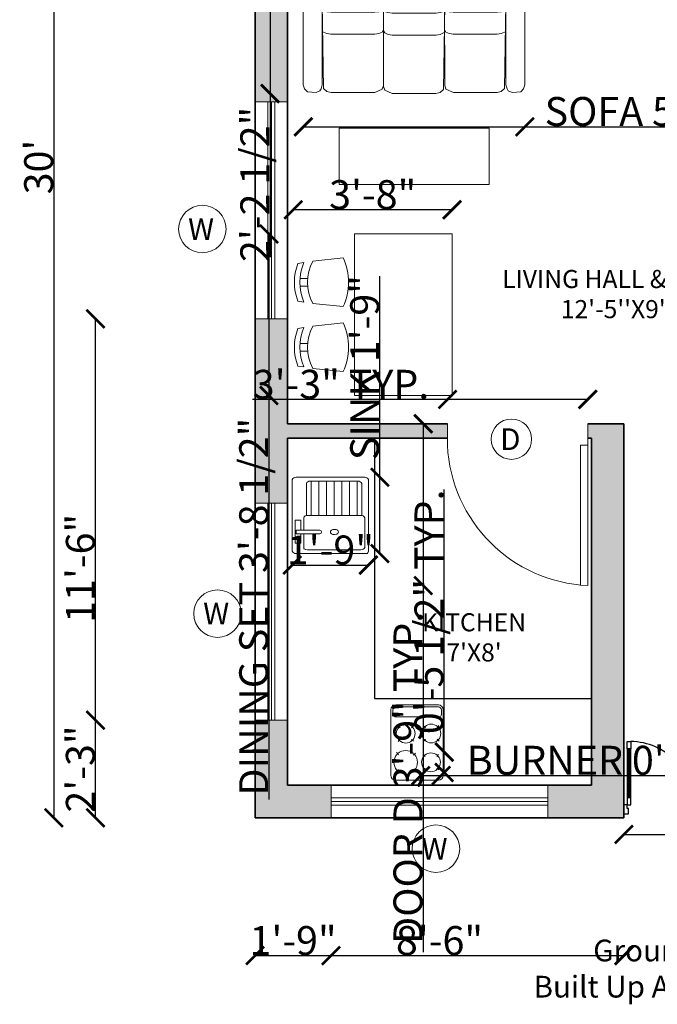
# Model space of a CAD drawing. Units: inches. Extents: x 2163 to 2555, y 1763 to 2232.
# Tile 1 of 3: x 2163 to 2339, y 1763 to 2035. Entities that reach past the tile are written whole.
import ezdxf

# ---------------------------------------------------------------- set-up
doc = ezdxf.new("R2010")
doc.units = ezdxf.units.IN
for name, color, linetype, lineweight in [('A-ANNO-DIMS', 2, 'Continuous', 18), ('A-ANNO-SYMB', 7, 'Continuous', 18), ('A-ANNO-TEXT', 7, 'Continuous', 18), ('A-AREA-IDEN', 7, 'Continuous', 18), ('A-EQPM', 9, 'Continuous', 18), ('A-FLOR-FIXT', 9, 'Continuous', 18), ('A-FURN', 8, 'Continuous', 18), ('A-WALL-PATT', 8, 'Continuous', 13), ('Doors', 222, 'Continuous', 18), ('Kitchen', 92, 'Continuous', 25), ('Walls', 7, 'Continuous', 35), ('Windows', 150, 'Continuous', 18)]:
    doc.layers.add(name, color=color, linetype=linetype, lineweight=lineweight)
doc.layers.add('A-Glaz', color=92, linetype='Continuous')
doc.layers.add('Main Door', color=150, linetype='Continuous')
doc.styles.get("Standard").update_dxf_attribs({"font": 'arial.ttf'})
doc.dimstyles.get("Standard").update_dxf_attribs({"dimtxt": 8, "dimasz": 5, "dimexe": 0.18, "dimexo": 0.0625, "dimgap": 0.09, "dimtad": 1, "dimdec": 1, "dimzin": 0, "dimdsep": 46, "dimlunit": 4, "dimtxsty": 'Standard', "dimblk": 'ARCHTICK', "dimcen": 0.09, "dimse1": 1, "dimse2": 1, "dimadec": 0, "dimazin": 0, "dimtfac": 1, "dimtdec": 1, "dimtofl": 0, "dimtmove": 0, "dimatfit": 3, "dimfxl": 1, "dimtolj": 1, "dimtzin": 0, "dimarcsym": 0})

# ---------------------------------------------------------------- blocks, each defined once
blk = doc.blocks.new('A$C13CE0A17')
at = {"layer": 'A-Glaz'}
for p, q in [((0.01, 0.61), (0.01, 0.08)), ((0.03, 0.08), (0.03, 0.61))]:
    blk.add_line(p, q, dxfattribs=at)
blk.add_lwpolyline([(1.4, 0.08), (1.4, 0.61), (1.42, 0.61), (1.42, 0.08)], close=True, dxfattribs=at)
at = {"layer": 'Main Door'}
for p, q in [((0, 0.61), (0, 0.69)), ((0, 0.69), (0.04, 0.69)), ((0.04, 0.69), (0.04, 0.61)), ((0, 0.61), (0, 0.08)), ((0.04, 0.61), (0, 0.61)), ((0.04, 0.61), (0, 0.61)), ((0.03, 0.61), (0.01, 0.61)), ((0.04, 0.08), (0.04, 0.61)), ((-0.035, 0), (-0.035, -0.1)), ((0, 0), (-0.035, 0)), ((0, 0.08), (0, 0)), ((0.04, 0.08), (0, 0.08)), ((0, 0.08), (0.04, 0.08)), ((0, 0), (0.04, 0)), ((0, -0.04), (0, 0)), ((0.01, 0.08), (0.03, 0.08)), ((0.04, 0), (0.04, 0.08)), ((-0.035, -0.1), (0.015, -0.1)), ((0.015, -0.04), (0, -0.04)), ((0.015, -0.05), (0.015, -0.04)), ((0.015, -0.1), (0.015, -0.05))]:
    blk.add_line(p, q, dxfattribs=at)
for points in [[(1.39, 0.69), (1.39, 0.61), (1.43, 0.61), (1.43, 0.69)], [(1.39, 0.08), (1.39, 0.61), (1.43, 0.61), (1.43, 0.08)], [(1.39, 0), (1.39, 0.08), (1.43, 0.08), (1.43, 0)], [(1.43, 0), (1.465, 0), (1.465, -0.1), (1.415, -0.1), (1.415, -0.05), (1.415, -0.04), (1.43, -0.04)]]:
    blk.add_lwpolyline(points, close=True, dxfattribs=at)
blk.add_arc((1.387, 0.017), 0.673, 89.7657, 181.4438, dxfattribs=at)
blk.add_ellipse((0.039, 0.051), major_axis=(0.667, -0.122), ratio=0.940794, start_param=0.11153, end_param=1.73917, dxfattribs=at)
blk = doc.blocks.new('S_SINK12')
for p, q in [((0.25, 0.45), (0.25, 0)), ((0.35, 0.45), (0.35, 0)), ((0.45, 0.45), (0.45, 0)), ((0.55, 0.45), (0.55, 0)), ((0.65, 0.45), (0.65, 0)), ((0.75, 0.45), (0.75, 0)), ((0.85, 0.45), (0.85, 0))]:
    blk.add_line(p, q)
for points in [[(0, -0.469), (0, 0.469, -0.310961), (0.05, 0.5), (0.95, 0.5, -0.310466), (1, 0.469), (1, -0.469, -0.414214), (0.969, -0.5), (0.05, -0.5, -0.309971)], [(0.052, -0.195), (0.052, -0.242), (0.362, -0.242, 1), (0.362, -0.195)], [(0.5, -0.217), (0.503, -0.229, 0.107136), (0.516, -0.241, 0.076468), (0.534, -0.249), (0.554, -0.251), (0.575, -0.248, 0.076468), (0.592, -0.241, 0.107136), (0.604, -0.229), (0.608, -0.217), (0.604, -0.205, 0.107136), (0.592, -0.193, 0.076468), (0.575, -0.186), (0.554, -0.183), (0.532, -0.186, 0.076468), (0.516, -0.193, 0.107136), (0.503, -0.205)]]:
    blk.add_lwpolyline(points, format="xyb", close=True)
for points in [[(0.185, -0.001), (0.185, 0.419, -0.310466), (0.235, 0.45), (0.862, 0.45, -0.310466), (0.912, 0.419), (0.912, 0, -0.310466)], [(0.15, -0.195), (0.15, -0.031, -0.310466), (0.2, 0), (0.9, 0, -0.310466), (0.95, -0.031), (0.95, -0.419, -0.310466), (0.9, -0.45), (0.2, -0.45), (0.18, -0.448, -0.071009), (0.165, -0.442, -0.106323), (0.153, -0.432), (0.15, -0.422), (0.151, -0.419)]]:
    blk.add_lwpolyline(points, format="xyb")
for points in [[(0.114, -0.242), (0.114, -0.364), (0.039, -0.364), (0.039, -0.064), (0.114, -0.064), (0.114, -0.195)], [(0.15, -0.419), (0.15, -0.242)]]:
    blk.add_lwpolyline(points)
blk = doc.blocks.new('table-23')
at = {"color": 0, "linetype": 'ByBlock'}
for p, q in [((-0.9, -1.4923), (-0.9, 0)), ((-0.9, 0), (0, 0)), ((0, -1.4923), (0, 0)), ((0.1062, -0.2211), (0.3862, -0.2511)), ((0.4677, -0.2639), (0.5237, -0.2726)), ((0.5049, -0.4111), (0.4347, -0.4111)), ((0.5049, -0.4811), (0.4347, -0.4811)), ((0.4677, -0.6284), (0.5237, -0.6197)), ((0.1062, -0.6711), (0.3862, -0.6411)), ((0.1062, -0.8211), (0.3862, -0.8511)), ((0.4677, -0.8639), (0.5237, -0.8726)), ((0.5049, -1.0111), (0.4347, -1.0111)), ((0.5049, -1.0811), (0.4347, -1.0811)), ((0.1062, -1.2711), (0.3862, -1.2411)), ((0.4677, -1.2284), (0.5237, -1.2197)), ((-0.9, -1.4923), (0, -1.4923))]:
    blk.add_line(p, q, dxfattribs=at)
for centre, radius, start, end in [((0.5875, -0.4461), 0.5312, 154.94238, 205.05762), ((0.031, -0.4461), 0.4053, 331.23721, 28.76279), ((0.0558, -0.4461), 0.4505, 336.13443, 23.86557), ((0.0765, -0.4461), 0.4797, 338.78869, 21.21131), ((0.5875, -1.0461), 0.5312, 154.94238, 205.05762), ((0.031, -1.0461), 0.4053, 331.23721, 28.76279), ((0.0558, -1.0461), 0.4505, 336.13443, 23.86557), ((0.0765, -1.0461), 0.4797, 338.78869, 21.21131)]:
    blk.add_arc(centre, radius, start, end, dxfattribs=at)
blk = doc.blocks.new('AP0B05')
for p, q in [((35, 100), (35, 880)), ((75, 100), (75, 878.9)), ((35, 100), (35, -20)), ((815, 100), (815, -20))]:
    blk.add_line(p, q)
blk.add_lwpolyline([(35, 100), (75, 100)])
blk.add_arc((-2.4, 62.6), 818.3, 2.6212, 87.3788)
blk = doc.blocks.new('12PCOU17')
at = {"color": 0, "linetype": 'ByBlock'}
for points in [[(-34.71, 34.72), (-33.66, 34.31), (-3.27, 34.3), (-1.81, 34.76), (-1.05, 35.2), (-0.38, 36.65), (-0.61, 39.84), (-1.73, 40.94), (-3.27, 41.4), (-33.66, 41.4), (-34.95, 40.5), (-35.65, 39.02), (-35.49, 35.83), (-34.71, 34.72)], [(-1.89, 11.91), (-1.66, 11.91), (-0.35, 14.68), (-0.35, 31.05), (-0.74, 32.58), (-1.89, 33.83), (-33.63, 34.3), (-34.84, 33.63), (-35.43, 32.38), (-35.68, 31), (-35.68, 14.74), (-35.43, 13.36), (-34.66, 11.99), (-33.44, 11.43), (-3, 11.44), (-1.66, 11.91)], [(-31.25, 11.43), (-31.06, 11.84), (-30.6, 13.09), (-30.4, 14.62), (-30.4, 31.12), (-30.6, 32.65), (-31.06, 33.9), (-31.81, 34.3)], [(-23.84, 11.43), (-22.99, 11.9), (-22.46, 13.15), (-22.23, 14.67), (-22.23, 31.07), (-22.46, 32.59), (-22.99, 33.84), (-23.12, 34.3)], [(-1.54, -10.96), (-1.31, -10.96), (0, -8.19), (0, 8.19), (-0.39, 9.71), (-1.54, 10.96), (-33.28, 11.44), (-34.5, 10.77), (-35.08, 9.51), (-35.33, 8.14), (-35.33, -8.13), (-35.08, -9.51), (-34.31, -10.87), (-33.1, -11.44), (-2.65, -11.43), (-1.31, -10.96)], [(-30.9, -11.44), (-30.72, -11.02), (-30.25, -9.77), (-30.05, -8.25), (-30.05, 8.26), (-30.25, 9.78), (-30.72, 11.03), (-31.47, 11.44)], [(-23.49, -11.44), (-22.64, -10.96), (-22.11, -9.72), (-21.88, -8.19), (-21.88, 8.2), (-22.11, 9.73), (-22.64, 10.97), (-22.77, 11.44)], [(-1.89, -11.91), (-1.66, -11.91), (-0.35, -14.68), (-0.35, -31.05), (-0.74, -32.58), (-1.89, -33.83), (-33.63, -34.3), (-34.84, -33.63), (-35.43, -32.38), (-35.68, -31), (-35.68, -14.74), (-35.43, -13.36), (-34.66, -11.99), (-33.44, -11.43), (-3, -11.44), (-1.66, -11.91)], [(-31.25, -11.43), (-31.06, -11.84), (-30.6, -13.09), (-30.4, -14.62), (-30.4, -31.12), (-30.6, -32.65), (-31.06, -33.9), (-31.81, -34.3)], [(-23.84, -11.43), (-22.99, -11.9), (-22.46, -13.15), (-22.23, -14.67), (-22.23, -31.07), (-22.46, -32.59), (-22.99, -33.84), (-23.12, -34.3)], [(-34.71, -34.72), (-33.66, -34.31), (-3.27, -34.3), (-1.81, -34.76), (-1.05, -35.2), (-0.38, -36.65), (-0.61, -39.84), (-1.73, -40.94), (-3.27, -41.4), (-33.66, -41.4), (-34.95, -40.5), (-35.65, -39.02), (-35.49, -35.83), (-34.71, -34.72)]]:
    blk.add_lwpolyline(points, dxfattribs=at)
blk = doc.blocks.new('_ArchTick')
at = {"color": 0, "linetype": 'ByBlock', "const_width": 0.15}
blk.add_lwpolyline([(-0.5, -0.5), (0.5, 0.5)], dxfattribs=at)
blk = doc.blocks.new('*D12')
at = {"layer": 'A-ANNO-DIMS', "color": 0, "lineweight": -2, "transparency": 16777216}
blk.add_line((2172.33, 2174.5), (2172.33, 1814.5), dxfattribs=at)
at = {"layer": 'Defpoints', "color": 0, "transparency": 16777216}
for p in [(2228.01, 2174.5), (2172.33, 1814.5), (2228.01, 1814.5)]:
    blk.add_point(p, dxfattribs=at)
at = {"layer": 'A-ANNO-DIMS', "color": 0, "lineweight": -2, "transparency": 16777216, "xscale": 5, "yscale": 5, "zscale": 5}
for p, rotation in [((2172.33, 2174.5), 90), ((2172.33, 1814.5), 270)]:
    blk.add_blockref('_ArchTick', p, dxfattribs=dict(at, rotation=rotation))
at = {"layer": 'A-ANNO-DIMS', "color": 0, "transparency": 16777216, "insert": (2168.15, 1994.5), "char_height": 8, "attachment_point": 5, "rotation": 90}
blk.add_mtext("\\A1;30'", dxfattribs=at)
blk = doc.blocks.new('WIN-60IN')
for p, q in [((0, 5.5), (60, 5.5)), ((0, 4.5), (60, 4.5)), ((0, 3.5), (60, 3.5))]:
    blk.add_line(p, q)
blk.add_lwpolyline([(0, 9), (60, 9), (60, 0), (0, 0)], close=True)
blk = doc.blocks.new('TAG-WINDOW-W')
blk.add_circle((6.57, 6.57), 6.57)
blk.add_text('W', height=6).set_placement((2.61, 3.57))
blk = doc.blocks.new('TAG-DOOR-D')
blk.add_circle((5.58, 5.58), 5.58)
blk.add_text('D', height=6).set_placement((2.46, 2.58))
blk = doc.blocks.new('COOKTOP-BURNER')
for p, q in [((0.44, 4.72), (1.01, 4.18)), ((4.72, 4.76), (4.18, 4.18)), ((0.47, 0.44), (1.02, 1.01)), ((4.76, 0.47), (4.18, 1.02))]:
    blk.add_line(p, q)
for start, end in [(138.017, 221.983), (48.017, 131.983), (318.017, 41.983), (228.017, 311.983)]:
    blk.add_arc((2.6, 2.6), 2.6, start, end)
blk = doc.blocks.new('*D20')
at = {"layer": 'A-ANNO-DIMS', "color": 0, "lineweight": -2, "transparency": 16777216}
for p, q in [((2274.51, 1923.5), (2274.51, 1878.74)), ((2274.51, 1878.74), (2274.51, 1777.39))]:
    blk.add_line(p, q, dxfattribs=at)
at = {"layer": 'Defpoints', "color": 0, "transparency": 16777216}
for p in [(2281.23, 1923.5), (2274.51, 1878.74), (2281.23, 1878.74)]:
    blk.add_point(p, dxfattribs=at)
at = {"layer": 'A-ANNO-DIMS', "color": 0, "lineweight": -2, "transparency": 16777216, "xscale": 5, "yscale": 5, "zscale": 5}
for p, rotation in [((2274.51, 1923.5), 90), ((2274.51, 1878.74), 270)]:
    blk.add_blockref('_ArchTick', p, dxfattribs=dict(at, rotation=rotation))
at = {"layer": 'A-ANNO-DIMS', "color": 0, "transparency": 16777216, "insert": (2270.28, 1825.56), "char_height": 8, "attachment_point": 5, "rotation": 90}
blk.add_mtext('\\A1;DOOR D 3\'-9" TYP.', dxfattribs=at)
blk = doc.blocks.new('*D21')
at = {"layer": 'A-ANNO-DIMS', "color": 0, "lineweight": -2, "transparency": 16777216}
for p, q in [((2281.23, 1930.22), (2227.29, 1930.22)), ((2320.02, 1930.22), (2281.23, 1930.22))]:
    blk.add_line(p, q, dxfattribs=at)
at = {"layer": 'Defpoints', "color": 0, "transparency": 16777216}
for p in [(2281.23, 1930.22), (2281.23, 1923.5), (2320.02, 1923.5)]:
    blk.add_point(p, dxfattribs=at)
at = {"layer": 'A-ANNO-DIMS', "color": 0, "lineweight": -2, "transparency": 16777216, "xscale": 5, "yscale": 5, "zscale": 5, "rotation": 180}
blk.add_blockref('_ArchTick', (2281.23, 1930.22), dxfattribs=at)
at = {"layer": 'A-ANNO-DIMS', "color": 0, "lineweight": -2, "transparency": 16777216, "xscale": 5, "yscale": 5, "zscale": 5}
blk.add_blockref('_ArchTick', (2320.02, 1930.22), dxfattribs=at)
at = {"layer": 'A-ANNO-DIMS', "color": 0, "transparency": 16777216, "insert": (2251.76, 1934.4), "char_height": 8, "attachment_point": 5}
blk.add_mtext('\\A1;3\'-3" TYP.', dxfattribs=at)
blk = doc.blocks.new('*D24')
at = {"layer": 'A-ANNO-DIMS', "color": 0, "lineweight": -2, "transparency": 16777216}
for p, q in [((2273.83, 1826.19), (2279.47, 1826.19)), ((2279.47, 1826.19), (2402, 1826.19))]:
    blk.add_line(p, q, dxfattribs=at)
at = {"layer": 'Defpoints', "color": 0, "transparency": 16777216}
for p in [(2273.83, 1827.04), (2279.47, 1827.04), (2279.47, 1826.19)]:
    blk.add_point(p, dxfattribs=at)
at = {"layer": 'A-ANNO-DIMS', "color": 0, "lineweight": -2, "transparency": 16777216, "xscale": 5, "yscale": 5, "zscale": 5, "rotation": 180}
blk.add_blockref('_ArchTick', (2273.83, 1826.19), dxfattribs=at)
at = {"layer": 'A-ANNO-DIMS', "color": 0, "lineweight": -2, "transparency": 16777216, "xscale": 5, "yscale": 5, "zscale": 5}
blk.add_blockref('_ArchTick', (2279.47, 1826.19), dxfattribs=at)
at = {"layer": 'A-ANNO-DIMS', "color": 0, "transparency": 16777216, "insert": (2343.23, 1830.42), "char_height": 8, "attachment_point": 5}
blk.add_mtext('\\A1;BURNER 0\'-5 1/2" TYP.', dxfattribs=at)
blk = doc.blocks.new('*D25')
at = {"layer": 'A-ANNO-DIMS', "color": 0, "lineweight": -2, "transparency": 16777216}
for p, q in [((2280.31, 1832.68), (2280.31, 1905.27)), ((2280.31, 1827.04), (2280.31, 1832.68))]:
    blk.add_line(p, q, dxfattribs=at)
at = {"layer": 'Defpoints', "color": 0, "transparency": 16777216}
for p in [(2279.47, 1832.68), (2280.31, 1832.68), (2279.47, 1827.04)]:
    blk.add_point(p, dxfattribs=at)
at = {"layer": 'A-ANNO-DIMS', "color": 0, "lineweight": -2, "transparency": 16777216, "xscale": 5, "yscale": 5, "zscale": 5}
for p, rotation in [((2280.31, 1832.68), 90), ((2280.31, 1827.04), 270)]:
    blk.add_blockref('_ArchTick', p, dxfattribs=dict(at, rotation=rotation))
at = {"layer": 'A-ANNO-DIMS', "color": 0, "transparency": 16777216, "insert": (2276.09, 1871.47), "char_height": 8, "attachment_point": 5, "rotation": 90}
blk.add_mtext('\\A1;0\'-5 1/2" TYP.', dxfattribs=at)
blk = doc.blocks.new('*D32')
at = {"layer": 'A-ANNO-DIMS', "color": 0, "lineweight": -2, "transparency": 16777216}
for p, q in [((2330.01, 1809.91), (2368.01, 1809.91)), ((2368.01, 1809.91), (2471.65, 1809.91))]:
    blk.add_line(p, q, dxfattribs=at)
at = {"layer": 'Defpoints', "color": 0, "transparency": 16777216}
for p in [(2330.01, 1815.61), (2368.01, 1815.61), (2368.01, 1809.91)]:
    blk.add_point(p, dxfattribs=at)
at = {"layer": 'A-ANNO-DIMS', "color": 0, "lineweight": -2, "transparency": 16777216, "xscale": 5, "yscale": 5, "zscale": 5, "rotation": 180}
blk.add_blockref('_ArchTick', (2330.01, 1809.91), dxfattribs=at)
at = {"layer": 'A-ANNO-DIMS', "color": 0, "lineweight": -2, "transparency": 16777216, "xscale": 5, "yscale": 5, "zscale": 5}
blk.add_blockref('_ArchTick', (2368.01, 1809.91), dxfattribs=at)
at = {"layer": 'A-ANNO-DIMS', "color": 0, "transparency": 16777216, "insert": (2422.33, 1814.14), "char_height": 8, "attachment_point": 5}
blk.add_mtext('\\A1;ENTRY DOOR 3\'-2"', dxfattribs=at)
blk = doc.blocks.new('*D34')
at = {"layer": 'A-ANNO-DIMS', "color": 0, "lineweight": -2, "transparency": 16777216}
for p, q in [((2262.54, 1908.7), (2262.54, 1964.3)), ((2262.54, 1887.57), (2262.54, 1908.7))]:
    blk.add_line(p, q, dxfattribs=at)
at = {"layer": 'Defpoints', "color": 0, "transparency": 16777216}
for p in [(2259.37, 1908.7), (2262.54, 1908.7), (2259.37, 1887.57)]:
    blk.add_point(p, dxfattribs=at)
at = {"layer": 'A-ANNO-DIMS', "color": 0, "lineweight": -2, "transparency": 16777216, "xscale": 5, "yscale": 5, "zscale": 5}
for p, rotation in [((2262.54, 1908.7), 90), ((2262.54, 1887.57), 270)]:
    blk.add_blockref('_ArchTick', p, dxfattribs=dict(at, rotation=rotation))
at = {"layer": 'A-ANNO-DIMS', "color": 0, "transparency": 16777216, "insert": (2258.32, 1939), "char_height": 8, "attachment_point": 5, "rotation": 90}
blk.add_mtext('\\A1;SINK 1\'-9"', dxfattribs=at)
blk = doc.blocks.new('*D35')
at = {"layer": 'A-ANNO-DIMS', "color": 0, "lineweight": -2, "transparency": 16777216}
blk.add_line((2238.28, 1884.4), (2259.37, 1884.4), dxfattribs=at)
at = {"layer": 'Defpoints', "color": 0, "transparency": 16777216}
for p in [(2238.28, 1887.57), (2259.37, 1887.57), (2259.37, 1884.4)]:
    blk.add_point(p, dxfattribs=at)
at = {"layer": 'A-ANNO-DIMS', "color": 0, "lineweight": -2, "transparency": 16777216, "xscale": 5, "yscale": 5, "zscale": 5, "rotation": 180}
blk.add_blockref('_ArchTick', (2238.28, 1884.4), dxfattribs=at)
at = {"layer": 'A-ANNO-DIMS', "color": 0, "lineweight": -2, "transparency": 16777216, "xscale": 5, "yscale": 5, "zscale": 5}
blk.add_blockref('_ArchTick', (2259.37, 1884.4), dxfattribs=at)
at = {"layer": 'A-ANNO-DIMS', "color": 0, "transparency": 16777216, "insert": (2248.83, 1888.57), "char_height": 8, "attachment_point": 5}
blk.add_mtext('\\A1;1\'-9"', dxfattribs=at)
blk = doc.blocks.new('*D36')
at = {"layer": 'A-ANNO-DIMS', "color": 0, "lineweight": -2, "transparency": 16777216}
for p, q in [((2231.85, 1975.97), (2231.85, 1931.28)), ((2231.85, 1931.28), (2231.85, 1819.53))]:
    blk.add_line(p, q, dxfattribs=at)
at = {"layer": 'Defpoints', "color": 0, "transparency": 16777216}
for p in [(2238.56, 1975.97), (2231.85, 1931.28), (2238.56, 1931.28)]:
    blk.add_point(p, dxfattribs=at)
at = {"layer": 'A-ANNO-DIMS', "color": 0, "lineweight": -2, "transparency": 16777216, "xscale": 5, "yscale": 5, "zscale": 5}
for p, rotation in [((2231.85, 1975.97), 90), ((2231.85, 1931.28), 270)]:
    blk.add_blockref('_ArchTick', p, dxfattribs=dict(at, rotation=rotation))
at = {"layer": 'A-ANNO-DIMS', "color": 0, "transparency": 16777216, "insert": (2227.62, 1872.9), "char_height": 8, "attachment_point": 5, "rotation": 90}
blk.add_mtext('\\A1;DINING SET 3\'-8 1/2"', dxfattribs=at)
blk = doc.blocks.new('*D37')
at = {"layer": 'A-ANNO-DIMS', "color": 0, "lineweight": -2, "transparency": 16777216}
blk.add_line((2282.49, 1982.67), (2238.56, 1982.67), dxfattribs=at)
at = {"layer": 'Defpoints', "color": 0, "transparency": 16777216}
for p in [(2238.56, 1982.67), (2238.56, 1975.97), (2282.49, 1975.97)]:
    blk.add_point(p, dxfattribs=at)
at = {"layer": 'A-ANNO-DIMS', "color": 0, "lineweight": -2, "transparency": 16777216, "xscale": 5, "yscale": 5, "zscale": 5, "rotation": 180}
blk.add_blockref('_ArchTick', (2238.56, 1982.67), dxfattribs=at)
at = {"layer": 'A-ANNO-DIMS', "color": 0, "lineweight": -2, "transparency": 16777216, "xscale": 5, "yscale": 5, "zscale": 5}
blk.add_blockref('_ArchTick', (2282.49, 1982.67), dxfattribs=at)
at = {"layer": 'A-ANNO-DIMS', "color": 0, "transparency": 16777216, "insert": (2260.53, 1986.85), "char_height": 8, "attachment_point": 5}
blk.add_mtext('\\A1;3\'-8"', dxfattribs=at)
blk = doc.blocks.new('*D38')
at = {"layer": 'A-ANNO-DIMS', "color": 0, "lineweight": -2, "transparency": 16777216}
for p, q in [((2241.35, 2005.61), (2302.62, 2005.61)), ((2302.62, 2005.61), (2381.2, 2005.61))]:
    blk.add_line(p, q, dxfattribs=at)
at = {"layer": 'Defpoints', "color": 0, "transparency": 16777216}
for p in [(2241.35, 2014.8), (2302.62, 2014.8), (2302.62, 2005.61)]:
    blk.add_point(p, dxfattribs=at)
at = {"layer": 'A-ANNO-DIMS', "color": 0, "lineweight": -2, "transparency": 16777216, "xscale": 5, "yscale": 5, "zscale": 5, "rotation": 180}
blk.add_blockref('_ArchTick', (2241.35, 2005.61), dxfattribs=at)
at = {"layer": 'A-ANNO-DIMS', "color": 0, "lineweight": -2, "transparency": 16777216, "xscale": 5, "yscale": 5, "zscale": 5}
blk.add_blockref('_ArchTick', (2302.62, 2005.61), dxfattribs=at)
at = {"layer": 'A-ANNO-DIMS', "color": 0, "transparency": 16777216, "insert": (2344.41, 2009.84), "char_height": 8, "attachment_point": 5}
blk.add_mtext('\\A1;SOFA 5\'-1 1/2"', dxfattribs=at)
blk = doc.blocks.new('*D39')
at = {"layer": 'A-ANNO-DIMS', "color": 0, "lineweight": -2, "transparency": 16777216}
for p, q in [((2232.15, 2041.21), (2232.15, 2014.8)), ((2232.15, 2014.8), (2232.15, 1969.58))]:
    blk.add_line(p, q, dxfattribs=at)
at = {"layer": 'Defpoints', "color": 0, "transparency": 16777216}
for p in [(2241.35, 2041.21), (2232.15, 2014.8), (2241.35, 2014.8)]:
    blk.add_point(p, dxfattribs=at)
at = {"layer": 'A-ANNO-DIMS', "color": 0, "lineweight": -2, "transparency": 16777216, "xscale": 5, "yscale": 5, "zscale": 5}
for p, rotation in [((2232.15, 2041.21), 90), ((2232.15, 2014.8), 270)]:
    blk.add_blockref('_ArchTick', p, dxfattribs=dict(at, rotation=rotation))
at = {"layer": 'A-ANNO-DIMS', "color": 0, "transparency": 16777216, "insert": (2227.93, 1989.69), "char_height": 8, "attachment_point": 5, "rotation": 90}
blk.add_mtext('\\A1;2\'-2 1/2"', dxfattribs=at)
blk = doc.blocks.new('*D45')
at = {"layer": 'A-ANNO-DIMS', "color": 0, "lineweight": -2, "transparency": 16777216}
blk.add_line((2228.01, 1776.39), (2249.01, 1776.39), dxfattribs=at)
at = {"layer": 'Defpoints', "color": 0, "transparency": 16777216}
for p in [(2228.01, 1814.5), (2249.01, 1814.5), (2249.01, 1776.39)]:
    blk.add_point(p, dxfattribs=at)
at = {"layer": 'A-ANNO-DIMS', "color": 0, "lineweight": -2, "transparency": 16777216, "xscale": 5, "yscale": 5, "zscale": 5, "rotation": 180}
blk.add_blockref('_ArchTick', (2228.01, 1776.39), dxfattribs=at)
at = {"layer": 'A-ANNO-DIMS', "color": 0, "lineweight": -2, "transparency": 16777216, "xscale": 5, "yscale": 5, "zscale": 5}
blk.add_blockref('_ArchTick', (2249.01, 1776.39), dxfattribs=at)
at = {"layer": 'A-ANNO-DIMS', "color": 0, "transparency": 16777216, "insert": (2238.51, 1780.56), "char_height": 8, "attachment_point": 5}
blk.add_mtext('\\A1;1\'-9"', dxfattribs=at)
blk = doc.blocks.new('*D46')
at = {"layer": 'A-ANNO-DIMS', "color": 0, "lineweight": -2, "transparency": 16777216}
blk.add_line((2228.01, 1776.39), (2330.01, 1776.39), dxfattribs=at)
at = {"layer": 'Defpoints', "color": 0, "transparency": 16777216}
for p in [(2228.01, 1814.5), (2330.01, 1814.5), (2330.01, 1776.39)]:
    blk.add_point(p, dxfattribs=at)
at = {"layer": 'A-ANNO-DIMS', "color": 0, "lineweight": -2, "transparency": 16777216, "xscale": 5, "yscale": 5, "zscale": 5, "rotation": 180}
blk.add_blockref('_ArchTick', (2228.01, 1776.39), dxfattribs=at)
at = {"layer": 'A-ANNO-DIMS', "color": 0, "lineweight": -2, "transparency": 16777216, "xscale": 5, "yscale": 5, "zscale": 5}
blk.add_blockref('_ArchTick', (2330.01, 1776.39), dxfattribs=at)
at = {"layer": 'A-ANNO-DIMS', "color": 0, "transparency": 16777216, "insert": (2279.01, 1780.56), "char_height": 8, "attachment_point": 5}
blk.add_mtext('\\A1;8\'-6"', dxfattribs=at)
blk = doc.blocks.new('*D47')
at = {"layer": 'A-ANNO-DIMS', "color": 0, "lineweight": -2, "transparency": 16777216}
blk.add_line((2183.86, 1814.5), (2183.86, 1841.5), dxfattribs=at)
at = {"layer": 'Defpoints', "color": 0, "transparency": 16777216}
for p in [(2183.86, 1841.5), (2228.01, 1841.5), (2228.01, 1814.5)]:
    blk.add_point(p, dxfattribs=at)
at = {"layer": 'A-ANNO-DIMS', "color": 0, "lineweight": -2, "transparency": 16777216, "xscale": 5, "yscale": 5, "zscale": 5}
for p, rotation in [((2183.86, 1841.5), 90), ((2183.86, 1814.5), 270)]:
    blk.add_blockref('_ArchTick', p, dxfattribs=dict(at, rotation=rotation))
at = {"layer": 'A-ANNO-DIMS', "color": 0, "transparency": 16777216, "insert": (2179.68, 1828), "char_height": 8, "attachment_point": 5, "rotation": 90}
blk.add_mtext('\\A1;2\'-3"', dxfattribs=at)
blk = doc.blocks.new('*D48')
at = {"layer": 'A-ANNO-DIMS', "color": 0, "lineweight": -2, "transparency": 16777216}
blk.add_line((2183.86, 1814.5), (2183.86, 1952.5), dxfattribs=at)
at = {"layer": 'Defpoints', "color": 0, "transparency": 16777216}
for p in [(2183.86, 1952.5), (2228.01, 1952.5), (2228.01, 1814.5)]:
    blk.add_point(p, dxfattribs=at)
at = {"layer": 'A-ANNO-DIMS', "color": 0, "lineweight": -2, "transparency": 16777216, "xscale": 5, "yscale": 5, "zscale": 5}
for p, rotation in [((2183.86, 1952.5), 90), ((2183.86, 1814.5), 270)]:
    blk.add_blockref('_ArchTick', p, dxfattribs=dict(at, rotation=rotation))
at = {"layer": 'A-ANNO-DIMS', "color": 0, "transparency": 16777216, "insert": (2179.68, 1883.5), "char_height": 8, "attachment_point": 5, "rotation": 90}
blk.add_mtext('\\A1;11\'-6"', dxfattribs=at)
blk = doc.blocks.new('*D55')
at = {"layer": 'A-ANNO-DIMS', "color": 0, "lineweight": -2, "transparency": 16777216}
blk.add_line((2237.01, 2215.35), (2261.01, 2215.35), dxfattribs=at)
at = {"layer": 'Defpoints', "color": 0, "transparency": 16777216}
for p in [(2261.01, 2215.35), (2237.01, 1919.5), (2261.01, 1919.5)]:
    blk.add_point(p, dxfattribs=at)
at = {"layer": 'A-ANNO-DIMS', "color": 0, "lineweight": -2, "transparency": 16777216, "xscale": 5, "yscale": 5, "zscale": 5, "rotation": 180}
blk.add_blockref('_ArchTick', (2237.01, 2215.35), dxfattribs=at)
at = {"layer": 'A-ANNO-DIMS', "color": 0, "lineweight": -2, "transparency": 16777216, "xscale": 5, "yscale": 5, "zscale": 5}
blk.add_blockref('_ArchTick', (2261.01, 2215.35), dxfattribs=at)
at = {"layer": 'A-ANNO-DIMS', "color": 0, "transparency": 16777216, "insert": (2249.01, 2219.53), "char_height": 8, "attachment_point": 5}
blk.add_mtext('\\A1;2\'-0"', dxfattribs=at)
blk = doc.blocks.new('*D58')
at = {"layer": 'A-ANNO-DIMS', "color": 0, "lineweight": -2, "transparency": 16777216}
for p, q in [((2265.57, 2215.35), (2280.07, 2215.35)), ((2280.07, 2215.35), (2324.4, 2215.35))]:
    blk.add_line(p, q, dxfattribs=at)
at = {"layer": 'Defpoints', "color": 0, "transparency": 16777216}
for p in [(2280.07, 2215.35), (2265.57, 1844.36), (2280.07, 1844.36)]:
    blk.add_point(p, dxfattribs=at)
at = {"layer": 'A-ANNO-DIMS', "color": 0, "lineweight": -2, "transparency": 16777216, "xscale": 5, "yscale": 5, "zscale": 5, "rotation": 180}
blk.add_blockref('_ArchTick', (2265.57, 2215.35), dxfattribs=at)
at = {"layer": 'A-ANNO-DIMS', "color": 0, "lineweight": -2, "transparency": 16777216, "xscale": 5, "yscale": 5, "zscale": 5}
blk.add_blockref('_ArchTick', (2280.07, 2215.35), dxfattribs=at)
at = {"layer": 'A-ANNO-DIMS', "color": 0, "transparency": 16777216, "insert": (2304.73, 2219.58), "char_height": 8, "attachment_point": 5}
blk.add_mtext('\\A1;1\'-2 1/2"', dxfattribs=at)
blk = doc.blocks.new('*D59')
at = {"layer": 'A-ANNO-DIMS', "color": 0, "lineweight": -2, "transparency": 16777216}
blk.add_line((2509.31, 1824.94), (2509.31, 1845.73), dxfattribs=at)
at = {"layer": 'Defpoints', "color": 0, "transparency": 16777216}
for p in [(2278.7, 1845.73), (2509.31, 1845.73), (2278.7, 1824.94)]:
    blk.add_point(p, dxfattribs=at)
at = {"layer": 'A-ANNO-DIMS', "color": 0, "lineweight": -2, "transparency": 16777216, "xscale": 5, "yscale": 5, "zscale": 5}
for p, rotation in [((2509.31, 1845.73), 90), ((2509.31, 1824.94), 270)]:
    blk.add_blockref('_ArchTick', p, dxfattribs=dict(at, rotation=rotation))
at = {"layer": 'A-ANNO-DIMS', "color": 0, "transparency": 16777216, "insert": (2505.14, 1835.33), "char_height": 8, "attachment_point": 5, "rotation": 90}
blk.add_mtext('\\A1;1\'-9"', dxfattribs=at)

msp = doc.modelspace()

# ---------------------------------------------------------------- hatches: boundary and pattern name
at = {"layer": 'A-WALL-PATT', "transparency": 33554585}
h = msp.add_hatch(color=256, dxfattribs=at)
h.dxf.hatch_style = 1
h.paths.add_polyline_path([(2261.51, 2174.5), (2228.01, 2174.5), (2228.01, 2135.5), (2237.01, 2135.5), (2237.01, 2165.5), (2261.51, 2165.5)])
h.paths.add_polyline_path([(2237.01, 2075.5), (2228.01, 2075.5), (2228.01, 2012.5), (2237.01, 2012.5), (2237.01, 2041.5), (2306.96, 2041.5), (2306.96, 2045.5), (2237.01, 2045.5)])
h.paths.add_polyline_path([(2237.01, 1952.5), (2228.01, 1952.5), (2228.01, 1901.5), (2237.01, 1901.5), (2237.01, 1919.5), (2281.23, 1919.5), (2281.23, 1923.5), (2237.01, 1923.5)])
h.paths.add_polyline_path([(2237.01, 1841.5), (2228.01, 1841.5), (2228.01, 1814.5), (2249.01, 1814.5), (2249.01, 1823.5), (2237.01, 1823.5)])
h.paths.add_polyline_path([(2330.01, 1923.5), (2320.02, 1923.5), (2320.02, 1919.5), (2321.01, 1919.5), (2321.01, 1823.5), (2309.01, 1823.5), (2309.01, 1814.5), (2330.01, 1814.5)])
h.paths.add_polyline_path([(2468.01, 1855.84), (2459.01, 1855.84), (2459.01, 1823.5), (2368.01, 1823.5), (2368.01, 1814.5), (2468.01, 1814.5)])
h.paths.add_polyline_path([(2468.01, 1949.34), (2459.01, 1949.34), (2459.01, 1923.5), (2390.01, 1923.5), (2390.01, 2001.5), (2391.3, 2001.5), (2391.3, 2005.5), (2386.01, 2005.5), (2386.01, 1923.5), (2368.01, 1923.5), (2368.01, 1914.5), (2459.01, 1914.5), (2459.01, 1882.16), (2468.01, 1882.16)])
h.paths.add_polyline_path([(2468.01, 2077.97), (2459.01, 2077.97), (2459.01, 2045.5), (2389.06, 2045.5), (2389.06, 2041.5), (2459.01, 2041.5), (2459.01, 2005.5), (2423.94, 2005.5), (2423.94, 2001.5), (2459.01, 2001.5), (2459.01, 1975.66), (2468.01, 1975.66)])
h.paths.add_polyline_path([(2468.01, 2174.5), (2434.51, 2174.5), (2434.51, 2165.5), (2450.4, 2165.5), (2459.01, 2165.5), (2459.01, 2137.97), (2468.01, 2137.97)])

# ---------------------------------------------------------------- linework, layer by layer
at = {"layer": 'A-EQPM'}
for p, q in [((2265.57, 1844.36), (2265.57, 1826.3)), ((2266.11, 1844.36), (2266.11, 1842.99)), ((2278.7, 1845.73), (2266.93, 1845.73)), ((2278.7, 1845.18), (2266.93, 1845.18)), ((2279.52, 1842.99), (2279.52, 1844.36)), ((2280.07, 1826.3), (2280.07, 1844.36)), ((2266.66, 1842.45), (2278.97, 1842.45)), ((2267.1, 1832.53), (2267.71, 1831.88)), ((2272.33, 1832.43), (2271.69, 1831.83)), ((2267.01, 1827.29), (2267.65, 1827.9)), ((2272.24, 1827.2), (2271.63, 1827.84)), ((2266.93, 1824.94), (2278.7, 1824.94))]:
    msp.add_line(p, q, dxfattribs=at)
for centre, radius, start, end in [((2266.93, 1844.36), 1.37, 90, 180), ((2266.93, 1844.36), 0.821, 90, 180), ((2278.7, 1844.36), 1.37, 0, 90), ((2278.7, 1844.36), 0.821, 0, 90), ((2266.66, 1842.99), 0.547, 180, 270), ((2278.97, 1842.99), 0.547, 270, 0), ((2269.67, 1829.86), 3.26, 48.017, 131.983), ((2269.67, 1829.86), 3.26, 138.017, 221.983), ((2269.67, 1829.86), 3.26, 318.017, 41.983), ((2269.67, 1829.86), 3.26, 228.017, 311.983), ((2266.93, 1826.3), 1.37, 180, 270), ((2278.7, 1826.3), 1.37, 270, 0)]:
    msp.add_arc(centre, radius, start, end, dxfattribs=at)
at = {"layer": 'A-FURN'}
msp.add_lwpolyline([(2251.24, 2005.19), (2292.79, 2005.19), (2292.79, 1989.62), (2251.24, 1989.62)], close=True, dxfattribs=at)
at = {"layer": 'Kitchen'}
for p, q in [((2261.01, 1919.5), (2261.01, 1847.5)), ((2261.01, 1847.5), (2321.01, 1847.5))]:
    msp.add_line(p, q, dxfattribs=at)
at = {"layer": 'Walls'}
for p, q in [((2228.01, 2174.5), (2228.01, 1814.5)), ((2237.01, 2041.5), (2237.01, 1923.5)), ((2237.01, 1923.5), (2281.23, 1923.5)), ((2320.02, 1923.5), (2330.01, 1923.5)), ((2330.01, 1923.5), (2330.01, 1814.5)), ((2237.01, 1919.5), (2281.23, 1919.5)), ((2237.01, 1919.5), (2237.01, 1823.5)), ((2320.02, 1919.5), (2321.01, 1919.5)), ((2321.01, 1919.5), (2321.01, 1823.5)), ((2237.01, 1823.5), (2321.01, 1823.5)), ((2228.01, 1814.5), (2330.01, 1814.5))]:
    msp.add_line(p, q, dxfattribs=at)

# ---------------------------------------------------------------- block references
at = {"layer": 'A-ANNO-SYMB'}
for name, p in [('TAG-WINDOW-W', (2206.86, 1970.76)), ('TAG-DOOR-D', (2293.32, 1913.63)), ('TAG-WINDOW-W', (2211.04, 1864.41)), ('TAG-WINDOW-W', (2271.45, 1799.39))]:
    msp.add_blockref(name, p, dxfattribs=at)
at = {"layer": 'A-EQPM'}
for p, rotation in [((2267.08, 1840.4), 269.8006253091953), ((2274.14, 1840.43), 270.0000000001496)]:
    msp.add_blockref('COOKTOP-BURNER', p, dxfattribs=dict(at, rotation=rotation))
msp.add_blockref('COOKTOP-BURNER', (2274.05, 1827.26), dxfattribs=at)
at = {"layer": 'A-FLOR-FIXT', "xscale": 21.0913660363013, "yscale": 21.0913660363013, "zscale": 21.0913660363013}
msp.add_blockref('S_SINK12', (2238.28, 1898.14), dxfattribs=at)
at = {"layer": 'A-FURN'}
for name, p, xscale, yscale, zscale, rotation in [('12PCOU17', (2271.98, 2014.8), 0.7400239287503789, 0.7400239287503789, 0.7400239287503789, 270), ('table-23', (2255.54, 1931.28), 29.94773308272323, 29.94773308272323, 29.94773308272323, 180)]:
    msp.add_blockref(name, p, dxfattribs=dict(at, xscale=xscale, yscale=yscale, zscale=zscale, rotation=rotation))
at = {"layer": 'Doors', "xscale": 0.0497371052158267, "yscale": 0.0497371052158267, "zscale": 0.0497371052158267, "rotation": 180}
msp.add_blockref('AP0B05', (2321.76, 1922.51), dxfattribs=at)
at = {"layer": 'Doors', "xscale": 25.33333333333333, "yscale": 25.33333333333333, "zscale": 25.33333333333333}
msp.add_blockref('A$C13CE0A17', (2330.9, 1818.14), dxfattribs=at)
at = {"layer": 'Windows', "rotation": 89.99999999999918}
for p in [(2237.01, 1952.5), (2237.01, 1841.5)]:
    msp.add_blockref('WIN-60IN', p, dxfattribs=at)
at = {"layer": 'Windows'}
msp.add_blockref('WIN-60IN', (2249.01, 1814.5), dxfattribs=at)

# ---------------------------------------------------------------- texts
at = {"layer": 'A-ANNO-TEXT', "insert": (2275.16, 1780.81), "char_height": 6, "attachment_point": 1}
msp.add_mtext_dynamic_manual_height_columns('\\pxqc;Ground Floor Plan\\PBuilt Up Area : 600.00 Sq. ft', width=162.2537, gutter_width=78.9, heights=[32.47], dxfattribs=at)
at = {"layer": 'A-AREA-IDEN', "char_height": 5, "attachment_point": 1}
for s, width, heights, insert in [("\\pxqc;LIVING HALL & DINNING\\P12'-5''X9'-10''", 82.4336, [20.1], (2292.72, 1966.02)), ("\\pxqc;KITCHEN\\P7'X8'", 40.594, [0], (2268.26, 1871.08))]:
    msp.add_mtext_dynamic_manual_height_columns(s, width=width, gutter_width=12.5, heights=heights, dxfattribs=dict(at, insert=insert))

# ---------------------------------------------------------------- dimensions: what is measured, and where the dimension line sits
at = {"layer": 'A-ANNO-DIMS'}
for base, p1, p2, picture, middle in [((2280.07, 2215.35), (2265.57, 1844.36), (2280.07, 1844.36), '*D58', (2304.73, 2219.58)), ((2261.01, 2215.35), (2237.01, 1919.5), (2261.01, 1919.5), '*D55', (2249.01, 2219.53)), ((2259.37, 1884.4), (2238.28, 1887.57), (2259.37, 1887.57), '*D35', (2248.83, 1888.57)), ((2249.01, 1776.39), (2228.01, 1814.5), (2249.01, 1814.5), '*D45', (2238.51, 1780.56)), ((2330.01, 1776.39), (2228.01, 1814.5), (2330.01, 1814.5), '*D46', (2279.01, 1780.56))]:
    dim = msp.add_linear_dim(base=base, p1=p1, p2=p2, dimstyle='Standard', override={"dimdec": 1, "dimlfac": 1, "dimrnd": 0, "dimzin": 1, "dimdsep": 46, "dimlunit": 4, "dimfrac": 2}, dxfattribs=at)
    dim.commit()
    dim.dimension.update_dxf_attribs({"geometry": picture, "text_midpoint": middle})
for base, p1, p2, angle, override, picture, middle in [((2172.33, 1814.5), (2228.01, 2174.5), (2228.01, 1814.5), 90, {"dimclrd": 0, "dimclre": 0, "dimclrt": 0}, '*D12', (2168.15, 1994.5)), ((2232.15, 2014.8), (2241.35, 2041.21), (2241.35, 2014.8), 270, {"dimdec": 1, "dimlfac": 1, "dimrnd": 0, "dimzin": 1, "dimdsep": 46, "dimlunit": 4, "dimfrac": 2}, '*D39', (2227.93, 1989.69)), ((2238.56, 1982.67), (2282.49, 1975.97), (2238.56, 1975.97), 180, {"dimdec": 1, "dimlfac": 1, "dimrnd": 0, "dimzin": 1, "dimdsep": 46, "dimlunit": 4, "dimfrac": 2}, '*D37', (2260.53, 1986.85)), ((2183.86, 1952.5), (2228.01, 1814.5), (2228.01, 1952.5), 90, {"dimdec": 1, "dimlfac": 1, "dimrnd": 0, "dimzin": 1, "dimdsep": 46, "dimlunit": 4, "dimfrac": 2}, '*D48', (2179.68, 1883.5)), ((2509.31, 1845.73), (2278.7, 1824.94), (2278.7, 1845.73), 90, {"dimdec": 1, "dimlfac": 1, "dimrnd": 0, "dimzin": 1, "dimdsep": 46, "dimlunit": 4, "dimfrac": 2}, '*D59', (2505.14, 1835.33)), ((2183.86, 1841.5), (2228.01, 1814.5), (2228.01, 1841.5), 90, {"dimdec": 1, "dimlfac": 1, "dimrnd": 0, "dimzin": 1, "dimdsep": 46, "dimlunit": 4, "dimfrac": 2}, '*D47', (2179.68, 1828))]:
    dim = msp.add_linear_dim(base=base, p1=p1, p2=p2, angle=angle, dimstyle='Standard', override=override, dxfattribs=at)
    dim.commit()
    dim.dimension.update_dxf_attribs({"geometry": picture, "text_midpoint": middle})
for base, p1, p2, text, picture, middle in [((2302.62, 2005.61), (2241.35, 2014.8), (2302.62, 2014.8), 'SOFA <>', '*D38', (2344.41, 2009.84)), ((2279.47, 1826.19), (2273.83, 1827.04), (2279.47, 1827.04), 'BURNER <> TYP.', '*D24', (2343.23, 1830.42)), ((2368.01, 1809.91), (2330.01, 1815.61), (2368.01, 1815.61), 'ENTRY DOOR <>', '*D32', (2422.33, 1814.14))]:
    dim = msp.add_linear_dim(base=base, p1=p1, p2=p2, text=text, dimstyle='Standard', override={"dimdec": 1, "dimlfac": 1, "dimrnd": 0, "dimzin": 1, "dimdsep": 46, "dimlunit": 4, "dimfrac": 2}, dxfattribs=at)
    dim.commit()
    dim.dimension.update_dxf_attribs({"geometry": picture, "text_midpoint": middle})
for base, p1, p2, angle, text, picture, middle in [((2231.85, 1931.28), (2238.56, 1975.97), (2238.56, 1931.28), 270, 'DINING SET <>', '*D36', (2227.62, 1872.9)), ((2262.54, 1908.7), (2259.37, 1887.57), (2259.37, 1908.7), 90, 'SINK <>', '*D34', (2258.32, 1939)), ((2281.23, 1930.22), (2320.02, 1923.5), (2281.23, 1923.5), 180, '<> TYP.', '*D21', (2251.76, 1934.4)), ((2274.51, 1878.74), (2281.23, 1923.5), (2281.23, 1878.74), 270, 'DOOR D <> TYP.', '*D20', (2270.28, 1825.56)), ((2280.31, 1832.68), (2279.47, 1827.04), (2279.47, 1832.68), 90, '<> TYP.', '*D25', (2276.09, 1871.47))]:
    dim = msp.add_linear_dim(base=base, p1=p1, p2=p2, angle=angle, text=text, dimstyle='Standard', override={"dimdec": 1, "dimlfac": 1, "dimrnd": 0, "dimzin": 1, "dimdsep": 46, "dimlunit": 4, "dimfrac": 2}, dxfattribs=at)
    dim.commit()
    dim.dimension.update_dxf_attribs({"geometry": picture, "text_midpoint": middle})

doc.saveas('drawing.dxf')
